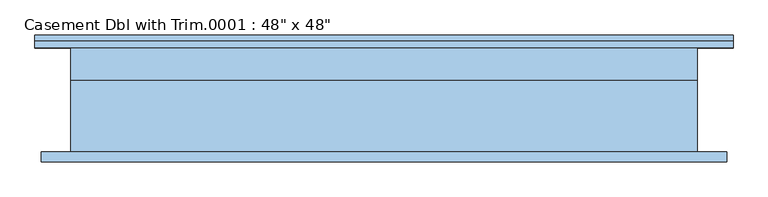
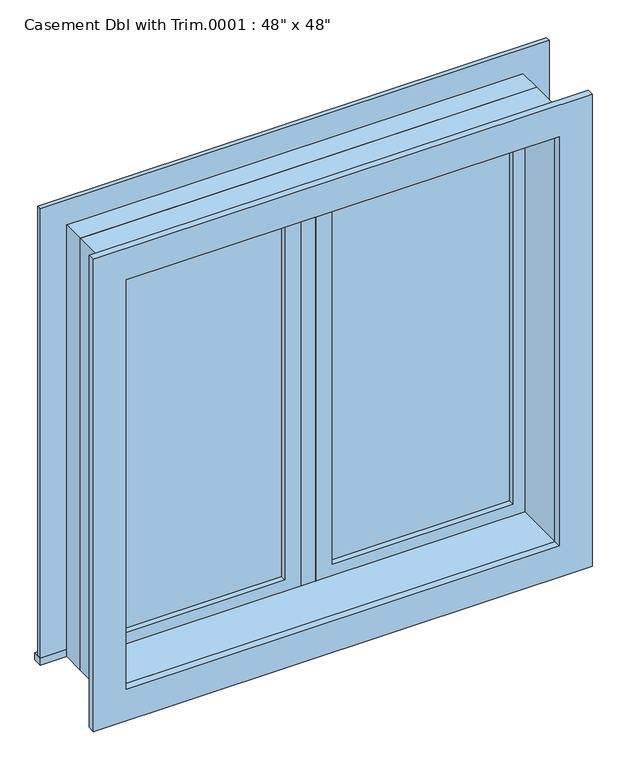
"""IFC4 building model written with IfcOpenShell, lengths in millimetres: window geometry."""

from ifc_helpers import new_model, si_unit, frame, origin, place, context, project, spatial, polyline, outline, extrude, source, transform, mapped, element, save


def window_0862ab64(model_context):
    return source(origin(), model_context, "Body", "SweptSolid", [
        extrude(outline(polyline([(63.5, 85.725), (546.1, 85.725), (546.1, 73.025), (63.5, 73.025), (63.5, 85.725)])), frame((0.0, 0.0, 977.9), z_axis=(0.0, 0.0, 1.0), x_axis=(1.0, 0.0, 0.0)), (0.0, 0.0, 1.0), 1092.2),
        extrude(outline(polyline([(2114.55, 19.05), (933.45, 19.05), (933.45, 590.55), (2114.55, 590.55), (2114.55, 19.05)]), holes=[polyline([(2070.1, 63.5), (2070.1, 546.1), (977.9, 546.1), (977.9, 63.5), (2070.1, 63.5)])]), frame((0.0, 57.15, 0.0), z_axis=(0.0, 1.0, 0.0), x_axis=(0.0, 0.0, 1.0)), (0.0, 0.0, 1.0), 44.45),
        extrude(outline(polyline([(19.05, 57.15), (-19.05, 57.15), (-19.05, 120.65), (19.05, 120.65), (19.05, 57.15)])), frame((0.0, 0.0, 933.45), z_axis=(0.0, 0.0, 1.0), x_axis=(1.0, 0.0, 0.0)), (0.0, 0.0, 1.0), 1181.1),
        extrude(outline(polyline([(-679.45, 146.05), (679.45, 146.05), (679.45, 120.65), (-679.45, 120.65), (-679.45, 146.05)])), frame((0.0, 0.0, 914.4), z_axis=(0.0, 0.0, 1.0), x_axis=(1.0, 0.0, 0.0)), (0.0, 0.0, 1.0), 19.05),
        extrude(outline(polyline([(2114.55, -590.55), (2114.55, 590.55), (933.45, 590.55), (933.45, 679.45), (2203.45, 679.45), (2203.45, -679.45), (933.45, -679.45), (933.45, -590.55), (2114.55, -590.55)])), frame((0.0, 120.65, 0.0), z_axis=(0.0, 1.0, 0.0), x_axis=(0.0, 0.0, 1.0)), (0.0, 0.0, 1.0), 12.7),
        extrude(outline(polyline([(2190.75, 666.75), (2190.75, -666.75), (857.25, -666.75), (857.25, 666.75), (2190.75, 666.75)]), holes=[polyline([(2101.85, 577.85), (946.15, 577.85), (946.15, -577.85), (2101.85, -577.85), (2101.85, 577.85)])]), frame((0.0, -101.6, 0.0), z_axis=(0.0, 1.0, 0.0), x_axis=(0.0, 0.0, 1.0)), (0.0, 0.0, 1.0), 19.05),
        extrude(outline(polyline([(-63.5, 73.025), (-546.1, 73.025), (-546.1, 85.725), (-63.5, 85.725), (-63.5, 73.025)])), frame((0.0, 0.0, 977.9), z_axis=(0.0, 0.0, 1.0), x_axis=(1.0, 0.0, 0.0)), (0.0, 0.0, 1.0), 1092.2),
        extrude(outline(polyline([(2114.55, -590.55), (933.45, -590.55), (933.45, -19.05), (2114.55, -19.05), (2114.55, -590.55)]), holes=[polyline([(2070.1, -546.1), (2070.1, -63.5), (977.9, -63.5), (977.9, -546.1), (2070.1, -546.1)])]), frame((0.0, 57.15, 0.0), z_axis=(0.0, 1.0, 0.0), x_axis=(0.0, 0.0, 1.0)), (0.0, 0.0, 1.0), 44.45),
        extrude(outline(polyline([(2133.6, -609.6), (914.4, -609.6), (914.4, 609.6), (2133.6, 609.6), (2133.6, -609.6)]), holes=[polyline([(2101.85, -577.85), (2101.85, 577.85), (946.15, 577.85), (946.15, -577.85), (2101.85, -577.85)])]), frame((0.0, -82.55, 0.0), z_axis=(0.0, 1.0, 0.0), x_axis=(0.0, 0.0, 1.0)), (0.0, 0.0, 1.0), 139.7),
        extrude(outline(polyline([(2133.6, 609.6), (2133.6, -609.6), (914.4, -609.6), (914.4, 609.6), (2133.6, 609.6)]), holes=[polyline([(2114.55, 590.55), (933.45, 590.55), (933.45, -590.55), (2114.55, -590.55), (2114.55, 590.55)])]), frame((0.0, 57.15, 0.0), z_axis=(0.0, 1.0, 0.0), x_axis=(0.0, 0.0, 1.0)), (0.0, 0.0, 1.0), 63.5),
    ])


if __name__ == "__main__":
    model = new_model("IFC4")
    model_context = context("Model", 3, world=origin())
    ifc_project = project(units=[si_unit("LENGTHUNIT", "METRE", prefix="MILLI")], contexts=[model_context])
    site = spatial("IfcSite", under=ifc_project)
    building = spatial("IfcBuilding", under=site)
    placement = place(None, origin())
    window_shape = window_0862ab64(model_context)
    element("IfcWindow", 1, ObjectType="Casement Dbl with Trim.0001 : 48\" x 48\"", at=placement, inside=building, context=model_context, shape_type="MappedRepresentation", body=[
        mapped(window_shape, transform((0.0, 0.0, 0.0), x_axis=(1.0, 0.0, 0.0), y_axis=(0.0, 1.0, 0.0), z_axis=(0.0, 0.0, 1.0))),
    ])
    save(model, "model.ifc")

# Revit data of these elements
# Type "Casement Dbl with Trim.0001 : 48\" x 48\""
#   Type Mark = "23"
#   Construction Type Id = "GSP4R"
#   Assembly Code = "B2020100"
#   Analytic Construction = "1/8 in Pilkington single glazing"
#   Visual Light Transmittance = 0.9
#   Solar Heat Gain Coefficient = 0.78
#   Heat Transfer Coefficient (U) = 0.6496 BTU/(h·ft²·°F)
#   Height = 4' - 0"
#   Default Sill Height = 3' - 0"
#   Trim Projection - Ext. = 0' - 0 1/2"
#   Trim Projection - Int. = 0' - 0 3/4"
#   Trim Width - Exterior = 0' - 3 1/2"
#   Trim Width - Interior = 0' - 3 1/2"
#   Width = 4' - 0"
#   Window Inset = 0' - 0 3/4"
#   Define Thermal Properties by = 1
#   Glass Pane Material = Glass
#   Sash Material = Sash
#   Trim Exterior Material = Trim
#   Trim Interior Material = Trim
#   Wall Closure = (empty or 0)
# Element 1 (IfcWindow, "Casement Dbl with Trim.0001 : 48\" x 48\"")
#   Materials on its faces: "Sash", "Trim", "Glass"
# Materials
#   "Glass": class "Glass", colour RGB 0 128 192, transparency 0.75, Description = "Soda Lime Glass", Cost = 0
#   "Sash": class "Wood", colour RGB 224 178 126, transparency 0
#   "Trim": class "Wood", colour RGB 224 178 126, transparency 0
